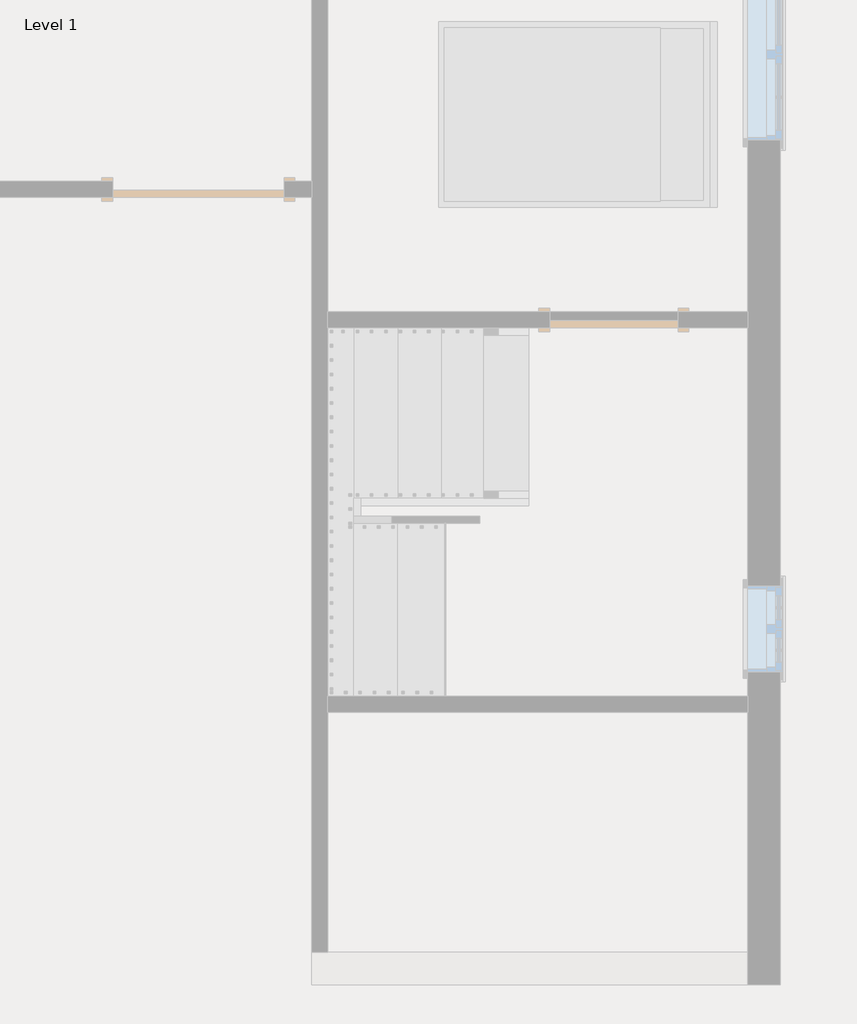
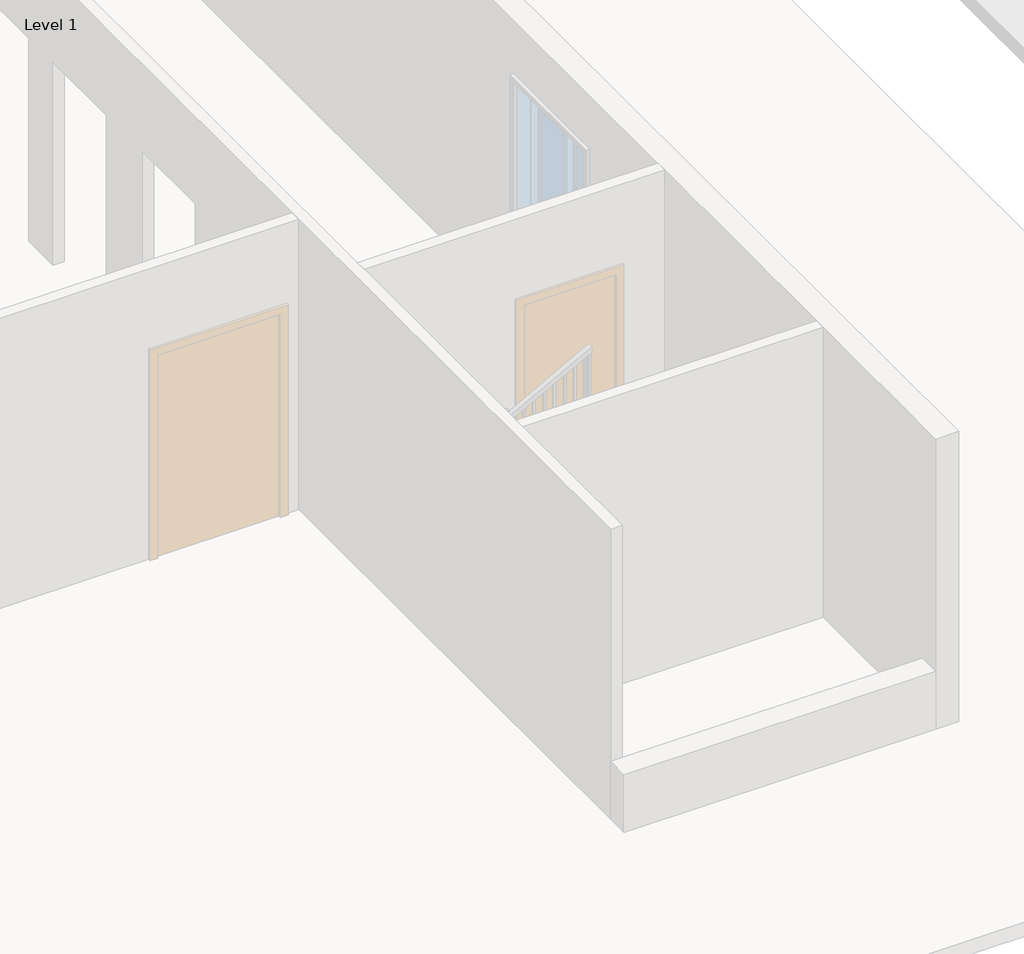
# One storey, part 6 of 7: 2 railings.
"""IFC4 building model written with IfcOpenShell, lengths in millimetres."""

from ifc_helpers import new_model, si_unit, frame, origin, place, context, project, spatial, polyline, outline, extrude, faceted_brep, element, save

model = new_model("IFC4")

# Units and contexts
model_context = context("Model", 3, world=origin())
ifc_project = project(units=[si_unit("LENGTHUNIT", "METRE", prefix="MILLI")], contexts=[model_context])

# Site, building, storey
site = spatial("IfcSite", under=ifc_project)
building = spatial("IfcBuilding", under=site)
storey = spatial("IfcBuildingStorey", under=building, Name="Level 1", Elevation=0.0)

# Railings
placement = place(None, origin())
element("IfcRailing", 1, ObjectType="Handrail - Rectangular", at=placement, inside=storey, context=model_context, shape_type="SolidModel", body=[
    faceted_brep([(7105.1820958, 5435.6, 1083.7333333), (7105.1820958, 5435.6, 1025.8977421), (7105.1820958, 5486.4, 1025.8977421), (7105.1820958, 5486.4, 1083.7333333), (5860.5820958, 5435.6, 1761.0666667), (5847.654197, 5435.6, 1710.2666667), (5847.654197, 5486.4, 1710.2666667), (5860.5820958, 5486.4, 1761.0666667), (5727.7, 5435.6, 1761.0666667), (5727.7, 5435.6, 1710.2666667), (5676.9, 5486.4, 1710.2666667), (5676.9, 5486.4, 1761.0666667), (5727.7, 2997.2, 1761.0666667), (5727.7, 2946.4, 1710.2666667), (5676.9, 2946.4, 1710.2666667), (5676.9, 2997.2, 1761.0666667), (5727.7, 2997.2, 1899.5526009), (5727.7, 2946.4, 1848.7526009), (5676.9, 2946.4, 1848.7526009), (5676.9, 2997.2, 1899.5526009), (5727.7, 2921.0, 1899.5526009), (5727.7, 2921.0, 1848.7526009), (5676.9, 2870.2, 1848.7526009), (5676.9, 2870.2, 1899.5526009), (5803.9, 2921.0, 1899.5526009), (5816.8278988, 2921.0, 1848.7526009), (5816.8278988, 2870.2, 1848.7526009), (5803.9, 2870.2, 1899.5526009), (7105.1820958, 2921.0, 2607.7333333), (7105.1820958, 2870.2, 2607.7333333), (7105.1820958, 2870.2, 2549.8977421), (7105.1820958, 2921.0, 2549.8977421)], [[[0, 1, 2, 3]], [[1, 0, 4, 5]], [[2, 1, 5, 6]], [[3, 2, 6, 7]], [[0, 3, 7, 4]], [[5, 4, 8, 9]], [[6, 5, 9, 10]], [[7, 6, 10, 11]], [[4, 7, 11, 8]], [[9, 8, 12, 13]], [[10, 9, 13, 14]], [[11, 10, 14, 15]], [[8, 11, 15, 12]], [[13, 12, 16, 17]], [[14, 13, 17, 18]], [[15, 14, 18, 19]], [[12, 15, 19, 16]], [[17, 16, 20, 21]], [[18, 17, 21, 22]], [[19, 18, 22, 23]], [[16, 19, 23, 20]], [[21, 20, 24, 25]], [[22, 21, 25, 26]], [[23, 22, 26, 27]], [[20, 23, 27, 24]], [[28, 29, 30, 31]], [[25, 24, 28, 31]], [[26, 25, 31, 30]], [[27, 26, 30, 29]], [[24, 27, 29, 28]]]),
    extrude(outline(polyline([(2510.4108873, 7032.625), (2500.0435403, 7013.575), (1524.0, 7013.575), (1524.0, 7032.625), (2510.4108873, 7032.625)])), frame((0.0, 2886.075, 0.0), z_axis=(0.0, 1.0, 0.0), x_axis=(0.0, 0.0, 1.0)), (0.0, 0.0, 1.0), 19.05),
    extrude(outline(polyline([(2455.1183703, 6931.025), (2444.7510233, 6911.975), (1524.0, 6911.975), (1524.0, 6931.025), (2455.1183703, 6931.025)])), frame((0.0, 2886.075, 0.0), z_axis=(0.0, 1.0, 0.0), x_axis=(0.0, 0.0, 1.0)), (0.0, 0.0, 1.0), 19.05),
    extrude(outline(polyline([(2399.8258533, 6829.425), (2389.4585063, 6810.375), (1524.0, 6810.375), (1524.0, 6829.425), (2399.8258533, 6829.425)])), frame((0.0, 2886.075, 0.0), z_axis=(0.0, 1.0, 0.0), x_axis=(0.0, 0.0, 1.0)), (0.0, 0.0, 1.0), 19.05),
    extrude(outline(polyline([(2344.5333363, 6727.825), (2334.1659893, 6708.775), (1354.6666667, 6708.775), (1354.6666667, 6727.825), (2344.5333363, 6727.825)])), frame((0.0, 2886.075, 0.0), z_axis=(0.0, 1.0, 0.0), x_axis=(0.0, 0.0, 1.0)), (0.0, 0.0, 1.0), 19.05),
    extrude(outline(polyline([(2289.2408192, 6626.225), (2278.8734723, 6607.175), (1354.6666667, 6607.175), (1354.6666667, 6626.225), (2289.2408192, 6626.225)])), frame((0.0, 2886.075, 0.0), z_axis=(0.0, 1.0, 0.0), x_axis=(0.0, 0.0, 1.0)), (0.0, 0.0, 1.0), 19.05),
    extrude(outline(polyline([(2233.9483022, 6524.625), (2223.5809553, 6505.575), (1354.6666667, 6505.575), (1354.6666667, 6524.625), (2233.9483022, 6524.625)])), frame((0.0, 2886.075, 0.0), z_axis=(0.0, 1.0, 0.0), x_axis=(0.0, 0.0, 1.0)), (0.0, 0.0, 1.0), 19.05),
    extrude(outline(polyline([(2178.6557852, 6423.025), (2168.2884383, 6403.975), (1185.3333333, 6403.975), (1185.3333333, 6423.025), (2178.6557852, 6423.025)])), frame((0.0, 2886.075, 0.0), z_axis=(0.0, 1.0, 0.0), x_axis=(0.0, 0.0, 1.0)), (0.0, 0.0, 1.0), 19.05),
    extrude(outline(polyline([(2123.3632682, 6321.425), (2112.9959213, 6302.375), (1185.3333333, 6302.375), (1185.3333333, 6321.425), (2123.3632682, 6321.425)])), frame((0.0, 2886.075, 0.0), z_axis=(0.0, 1.0, 0.0), x_axis=(0.0, 0.0, 1.0)), (0.0, 0.0, 1.0), 19.05),
    extrude(outline(polyline([(2068.0707512, 6219.825), (2057.7034043, 6200.775), (1185.3333333, 6200.775), (1185.3333333, 6219.825), (2068.0707512, 6219.825)])), frame((0.0, 2886.075, 0.0), z_axis=(0.0, 1.0, 0.0), x_axis=(0.0, 0.0, 1.0)), (0.0, 0.0, 1.0), 19.05),
    extrude(outline(polyline([(2012.7782342, 6118.225), (2002.4108873, 6099.175), (1016.0, 6099.175), (1016.0, 6118.225), (2012.7782342, 6118.225)])), frame((0.0, 2886.075, 0.0), z_axis=(0.0, 1.0, 0.0), x_axis=(0.0, 0.0, 1.0)), (0.0, 0.0, 1.0), 19.05),
    extrude(outline(polyline([(1957.4857172, 6016.625), (1947.1183703, 5997.575), (1016.0, 5997.575), (1016.0, 6016.625), (1957.4857172, 6016.625)])), frame((0.0, 2886.075, 0.0), z_axis=(0.0, 1.0, 0.0), x_axis=(0.0, 0.0, 1.0)), (0.0, 0.0, 1.0), 19.05),
    extrude(outline(polyline([(1902.1932002, 5915.025), (1891.8258533, 5895.975), (1016.0, 5895.975), (1016.0, 5915.025), (1902.1932002, 5915.025)])), frame((0.0, 2886.075, 0.0), z_axis=(0.0, 1.0, 0.0), x_axis=(0.0, 0.0, 1.0)), (0.0, 0.0, 1.0), 19.05),
    extrude(outline(polyline([(1846.9006832, 5813.425), (1836.5333363, 5794.375), (846.6666667, 5794.375), (846.6666667, 5813.425), (1846.9006832, 5813.425)])), frame((0.0, 2886.075, 0.0), z_axis=(0.0, 1.0, 0.0), x_axis=(0.0, 0.0, 1.0)), (0.0, 0.0, 1.0), 19.05),
    extrude(outline(polyline([(5692.775, 2930.525), (5711.825, 2930.525), (5711.825, 2911.475), (5692.775, 2911.475), (5692.775, 2930.525)])), frame((0.0, 0.0, 846.6666667), z_axis=(0.0, 0.0, 1.0), x_axis=(1.0, 0.0, 0.0)), (0.0, 0.0, 1.0), 1002.0859343),
    extrude(outline(polyline([(5692.775, 3032.125), (5711.825, 3032.125), (5711.825, 3013.075), (5692.775, 3013.075), (5692.775, 3032.125)])), frame((0.0, 0.0, 846.6666667), z_axis=(0.0, 0.0, 1.0), x_axis=(1.0, 0.0, 0.0)), (0.0, 0.0, 1.0), 863.6),
    extrude(outline(polyline([(5692.775, 3133.725), (5711.825, 3133.725), (5711.825, 3114.675), (5692.775, 3114.675), (5692.775, 3133.725)])), frame((0.0, 0.0, 846.6666667), z_axis=(0.0, 0.0, 1.0), x_axis=(1.0, 0.0, 0.0)), (0.0, 0.0, 1.0), 863.6),
    extrude(outline(polyline([(5692.775, 3235.325), (5711.825, 3235.325), (5711.825, 3216.275), (5692.775, 3216.275), (5692.775, 3235.325)])), frame((0.0, 0.0, 846.6666667), z_axis=(0.0, 0.0, 1.0), x_axis=(1.0, 0.0, 0.0)), (0.0, 0.0, 1.0), 863.6),
    extrude(outline(polyline([(5692.775, 3336.925), (5711.825, 3336.925), (5711.825, 3317.875), (5692.775, 3317.875), (5692.775, 3336.925)])), frame((0.0, 0.0, 846.6666667), z_axis=(0.0, 0.0, 1.0), x_axis=(1.0, 0.0, 0.0)), (0.0, 0.0, 1.0), 863.6),
    extrude(outline(polyline([(5692.775, 3438.525), (5711.825, 3438.525), (5711.825, 3419.475), (5692.775, 3419.475), (5692.775, 3438.525)])), frame((0.0, 0.0, 846.6666667), z_axis=(0.0, 0.0, 1.0), x_axis=(1.0, 0.0, 0.0)), (0.0, 0.0, 1.0), 863.6),
    extrude(outline(polyline([(5692.775, 3540.125), (5711.825, 3540.125), (5711.825, 3521.075), (5692.775, 3521.075), (5692.775, 3540.125)])), frame((0.0, 0.0, 846.6666667), z_axis=(0.0, 0.0, 1.0), x_axis=(1.0, 0.0, 0.0)), (0.0, 0.0, 1.0), 863.6),
    extrude(outline(polyline([(5692.775, 3641.725), (5711.825, 3641.725), (5711.825, 3622.675), (5692.775, 3622.675), (5692.775, 3641.725)])), frame((0.0, 0.0, 846.6666667), z_axis=(0.0, 0.0, 1.0), x_axis=(1.0, 0.0, 0.0)), (0.0, 0.0, 1.0), 863.6),
    extrude(outline(polyline([(5692.775, 3743.325), (5711.825, 3743.325), (5711.825, 3724.275), (5692.775, 3724.275), (5692.775, 3743.325)])), frame((0.0, 0.0, 846.6666667), z_axis=(0.0, 0.0, 1.0), x_axis=(1.0, 0.0, 0.0)), (0.0, 0.0, 1.0), 863.6),
    extrude(outline(polyline([(5692.775, 3844.925), (5711.825, 3844.925), (5711.825, 3825.875), (5692.775, 3825.875), (5692.775, 3844.925)])), frame((0.0, 0.0, 846.6666667), z_axis=(0.0, 0.0, 1.0), x_axis=(1.0, 0.0, 0.0)), (0.0, 0.0, 1.0), 863.6),
    extrude(outline(polyline([(5692.775, 3946.525), (5711.825, 3946.525), (5711.825, 3927.475), (5692.775, 3927.475), (5692.775, 3946.525)])), frame((0.0, 0.0, 846.6666667), z_axis=(0.0, 0.0, 1.0), x_axis=(1.0, 0.0, 0.0)), (0.0, 0.0, 1.0), 863.6),
    extrude(outline(polyline([(5692.775, 4048.125), (5711.825, 4048.125), (5711.825, 4029.075), (5692.775, 4029.075), (5692.775, 4048.125)])), frame((0.0, 0.0, 846.6666667), z_axis=(0.0, 0.0, 1.0), x_axis=(1.0, 0.0, 0.0)), (0.0, 0.0, 1.0), 863.6),
    extrude(outline(polyline([(5692.775, 4149.725), (5711.825, 4149.725), (5711.825, 4130.675), (5692.775, 4130.675), (5692.775, 4149.725)])), frame((0.0, 0.0, 846.6666667), z_axis=(0.0, 0.0, 1.0), x_axis=(1.0, 0.0, 0.0)), (0.0, 0.0, 1.0), 863.6),
    extrude(outline(polyline([(5692.775, 4251.325), (5711.825, 4251.325), (5711.825, 4232.275), (5692.775, 4232.275), (5692.775, 4251.325)])), frame((0.0, 0.0, 846.6666667), z_axis=(0.0, 0.0, 1.0), x_axis=(1.0, 0.0, 0.0)), (0.0, 0.0, 1.0), 863.6),
    extrude(outline(polyline([(5692.775, 4352.925), (5711.825, 4352.925), (5711.825, 4333.875), (5692.775, 4333.875), (5692.775, 4352.925)])), frame((0.0, 0.0, 846.6666667), z_axis=(0.0, 0.0, 1.0), x_axis=(1.0, 0.0, 0.0)), (0.0, 0.0, 1.0), 863.6),
    extrude(outline(polyline([(5692.775, 4454.525), (5711.825, 4454.525), (5711.825, 4435.475), (5692.775, 4435.475), (5692.775, 4454.525)])), frame((0.0, 0.0, 846.6666667), z_axis=(0.0, 0.0, 1.0), x_axis=(1.0, 0.0, 0.0)), (0.0, 0.0, 1.0), 863.6),
    extrude(outline(polyline([(5692.775, 4556.125), (5711.825, 4556.125), (5711.825, 4537.075), (5692.775, 4537.075), (5692.775, 4556.125)])), frame((0.0, 0.0, 846.6666667), z_axis=(0.0, 0.0, 1.0), x_axis=(1.0, 0.0, 0.0)), (0.0, 0.0, 1.0), 863.6),
    extrude(outline(polyline([(5692.775, 4657.725), (5711.825, 4657.725), (5711.825, 4638.675), (5692.775, 4638.675), (5692.775, 4657.725)])), frame((0.0, 0.0, 846.6666667), z_axis=(0.0, 0.0, 1.0), x_axis=(1.0, 0.0, 0.0)), (0.0, 0.0, 1.0), 863.6),
    extrude(outline(polyline([(5692.775, 4759.325), (5711.825, 4759.325), (5711.825, 4740.275), (5692.775, 4740.275), (5692.775, 4759.325)])), frame((0.0, 0.0, 846.6666667), z_axis=(0.0, 0.0, 1.0), x_axis=(1.0, 0.0, 0.0)), (0.0, 0.0, 1.0), 863.6),
    extrude(outline(polyline([(5692.775, 4860.925), (5711.825, 4860.925), (5711.825, 4841.875), (5692.775, 4841.875), (5692.775, 4860.925)])), frame((0.0, 0.0, 846.6666667), z_axis=(0.0, 0.0, 1.0), x_axis=(1.0, 0.0, 0.0)), (0.0, 0.0, 1.0), 863.6),
    extrude(outline(polyline([(5692.775, 4962.525), (5711.825, 4962.525), (5711.825, 4943.475), (5692.775, 4943.475), (5692.775, 4962.525)])), frame((0.0, 0.0, 846.6666667), z_axis=(0.0, 0.0, 1.0), x_axis=(1.0, 0.0, 0.0)), (0.0, 0.0, 1.0), 863.6),
    extrude(outline(polyline([(5692.775, 5064.125), (5711.825, 5064.125), (5711.825, 5045.075), (5692.775, 5045.075), (5692.775, 5064.125)])), frame((0.0, 0.0, 846.6666667), z_axis=(0.0, 0.0, 1.0), x_axis=(1.0, 0.0, 0.0)), (0.0, 0.0, 1.0), 863.6),
    extrude(outline(polyline([(5692.775, 5165.725), (5711.825, 5165.725), (5711.825, 5146.675), (5692.775, 5146.675), (5692.775, 5165.725)])), frame((0.0, 0.0, 846.6666667), z_axis=(0.0, 0.0, 1.0), x_axis=(1.0, 0.0, 0.0)), (0.0, 0.0, 1.0), 863.6),
    extrude(outline(polyline([(5692.775, 5267.325), (5711.825, 5267.325), (5711.825, 5248.275), (5692.775, 5248.275), (5692.775, 5267.325)])), frame((0.0, 0.0, 846.6666667), z_axis=(0.0, 0.0, 1.0), x_axis=(1.0, 0.0, 0.0)), (0.0, 0.0, 1.0), 863.6),
    extrude(outline(polyline([(5692.775, 5368.925), (5711.825, 5368.925), (5711.825, 5349.875), (5692.775, 5349.875), (5692.775, 5368.925)])), frame((0.0, 0.0, 846.6666667), z_axis=(0.0, 0.0, 1.0), x_axis=(1.0, 0.0, 0.0)), (0.0, 0.0, 1.0), 863.6),
    extrude(outline(polyline([(5793.9070958, 5470.525), (5793.9070958, 5451.475), (5774.8570958, 5451.475), (5774.8570958, 5470.525), (5793.9070958, 5470.525)])), frame((0.0, 0.0, 846.6666667), z_axis=(0.0, 0.0, 1.0), x_axis=(1.0, 0.0, 0.0)), (0.0, 0.0, 1.0), 863.6),
    extrude(outline(polyline([(1684.2242727, 5895.5070958), (1694.5916197, 5876.4570958), (677.3333333, 5876.4570958), (677.3333333, 5895.5070958), (1684.2242727, 5895.5070958)])), frame((0.0, 5451.475, 0.0), z_axis=(0.0, 1.0, 0.0), x_axis=(0.0, 0.0, 1.0)), (0.0, 0.0, 1.0), 19.05),
    extrude(outline(polyline([(1628.9317557, 5997.1070958), (1639.2991027, 5978.0570958), (677.3333333, 5978.0570958), (677.3333333, 5997.1070958), (1628.9317557, 5997.1070958)])), frame((0.0, 5451.475, 0.0), z_axis=(0.0, 1.0, 0.0), x_axis=(0.0, 0.0, 1.0)), (0.0, 0.0, 1.0), 19.05),
    extrude(outline(polyline([(1573.6392387, 6098.7070958), (1584.0065857, 6079.6570958), (677.3333333, 6079.6570958), (677.3333333, 6098.7070958), (1573.6392387, 6098.7070958)])), frame((0.0, 5451.475, 0.0), z_axis=(0.0, 1.0, 0.0), x_axis=(0.0, 0.0, 1.0)), (0.0, 0.0, 1.0), 19.05),
    extrude(outline(polyline([(1518.3467217, 6200.3070958), (1528.7140687, 6181.2570958), (508.0, 6181.2570958), (508.0, 6200.3070958), (1518.3467217, 6200.3070958)])), frame((0.0, 5451.475, 0.0), z_axis=(0.0, 1.0, 0.0), x_axis=(0.0, 0.0, 1.0)), (0.0, 0.0, 1.0), 19.05),
    extrude(outline(polyline([(1463.0542047, 6301.9070958), (1473.4215517, 6282.8570958), (508.0, 6282.8570958), (508.0, 6301.9070958), (1463.0542047, 6301.9070958)])), frame((0.0, 5451.475, 0.0), z_axis=(0.0, 1.0, 0.0), x_axis=(0.0, 0.0, 1.0)), (0.0, 0.0, 1.0), 19.05),
    extrude(outline(polyline([(1407.7616877, 6403.5070958), (1418.1290347, 6384.4570958), (508.0, 6384.4570958), (508.0, 6403.5070958), (1407.7616877, 6403.5070958)])), frame((0.0, 5451.475, 0.0), z_axis=(0.0, 1.0, 0.0), x_axis=(0.0, 0.0, 1.0)), (0.0, 0.0, 1.0), 19.05),
    extrude(outline(polyline([(1352.4691707, 6505.1070958), (1362.8365176, 6486.0570958), (338.6666667, 6486.0570958), (338.6666667, 6505.1070958), (1352.4691707, 6505.1070958)])), frame((0.0, 5451.475, 0.0), z_axis=(0.0, 1.0, 0.0), x_axis=(0.0, 0.0, 1.0)), (0.0, 0.0, 1.0), 19.05),
    extrude(outline(polyline([(1297.1766537, 6606.7070958), (1307.5440006, 6587.6570958), (338.6666667, 6587.6570958), (338.6666667, 6606.7070958), (1297.1766537, 6606.7070958)])), frame((0.0, 5451.475, 0.0), z_axis=(0.0, 1.0, 0.0), x_axis=(0.0, 0.0, 1.0)), (0.0, 0.0, 1.0), 19.05),
    extrude(outline(polyline([(1241.8841367, 6708.3070958), (1252.2514836, 6689.2570958), (338.6666667, 6689.2570958), (338.6666667, 6708.3070958), (1241.8841367, 6708.3070958)])), frame((0.0, 5451.475, 0.0), z_axis=(0.0, 1.0, 0.0), x_axis=(0.0, 0.0, 1.0)), (0.0, 0.0, 1.0), 19.05),
    extrude(outline(polyline([(1186.5916197, 6809.9070958), (1196.9589666, 6790.8570958), (169.3333333, 6790.8570958), (169.3333333, 6809.9070958), (1186.5916197, 6809.9070958)])), frame((0.0, 5451.475, 0.0), z_axis=(0.0, 1.0, 0.0), x_axis=(0.0, 0.0, 1.0)), (0.0, 0.0, 1.0), 19.05),
    extrude(outline(polyline([(1131.2991027, 6911.5070958), (1141.6664496, 6892.4570958), (169.3333333, 6892.4570958), (169.3333333, 6911.5070958), (1131.2991027, 6911.5070958)])), frame((0.0, 5451.475, 0.0), z_axis=(0.0, 1.0, 0.0), x_axis=(0.0, 0.0, 1.0)), (0.0, 0.0, 1.0), 19.05),
    extrude(outline(polyline([(1076.0065857, 7013.1070958), (1086.3739326, 6994.0570958), (169.3333333, 6994.0570958), (169.3333333, 7013.1070958), (1076.0065857, 7013.1070958)])), frame((0.0, 5451.475, 0.0), z_axis=(0.0, 1.0, 0.0), x_axis=(0.0, 0.0, 1.0)), (0.0, 0.0, 1.0), 19.05),
    extrude(outline(polyline([(5692.775, 2905.125), (5711.825, 2905.125), (5711.825, 2886.075), (5692.775, 2886.075), (5692.775, 2905.125)])), frame((0.0, 0.0, 846.6666667), z_axis=(0.0, 0.0, 1.0), x_axis=(1.0, 0.0, 0.0)), (0.0, 0.0, 1.0), 1002.0859343),
    extrude(outline(polyline([(5711.825, 5470.525), (5711.825, 5451.475), (5692.775, 5451.475), (5692.775, 5470.525), (5711.825, 5470.525)])), frame((0.0, 0.0, 846.6666667), z_axis=(0.0, 0.0, 1.0), x_axis=(1.0, 0.0, 0.0)), (0.0, 0.0, 1.0), 863.6),
    extrude(outline(polyline([(2549.8977421, 7105.1820958), (2539.5303952, 7086.1320958), (1524.0, 7086.1320958), (1524.0, 7105.1820958), (2549.8977421, 7105.1820958)])), frame((0.0, 2886.075, 0.0), z_axis=(0.0, 1.0, 0.0), x_axis=(0.0, 0.0, 1.0)), (0.0, 0.0, 1.0), 19.05),
    extrude(outline(polyline([(1025.8977421, 7105.1820958), (1036.2650891, 7086.1320958), (169.3333333, 7086.1320958), (169.3333333, 7105.1820958), (1025.8977421, 7105.1820958)])), frame((0.0, 5451.475, 0.0), z_axis=(0.0, 1.0, 0.0), x_axis=(0.0, 0.0, 1.0)), (0.0, 0.0, 1.0), 19.05),
])
element("IfcRailing", 2, ObjectType="Handrail - Rectangular", at=placement, inside=storey, context=model_context, shape_type="SolidModel", body=[
    faceted_brep([(7105.1820958, 4274.6882626, 1083.7333333), (7105.1820958, 4274.6882626, 1025.8977421), (7105.1820958, 4325.4882626, 1025.8977421), (7105.1820958, 4325.4882626, 1083.7333333), (5936.7820958, 4274.6882626, 1719.5972789), (5885.9820958, 4274.6882626, 1689.4079462), (5885.9820958, 4325.4882626, 1689.4079462), (5936.7820958, 4325.4882626, 1719.5972789), (5936.7820958, 4274.6882626, 1761.0666667), (5885.9820958, 4274.6882626, 1710.2666667), (5885.9820958, 4325.4882626, 1710.2666667), (5936.7820958, 4325.4882626, 1761.0666667), (5860.5820958, 4274.6882626, 1761.0666667), (5860.5820958, 4274.6882626, 1710.2666667), (5809.7820958, 4325.4882626, 1710.2666667), (5809.7820958, 4325.4882626, 1761.0666667), (5860.5820958, 4198.4882626, 1761.0666667), (5860.5820958, 4198.4882626, 1710.2666667), (5809.7820958, 4198.4882626, 1710.2666667), (5809.7820958, 4198.4882626, 1761.0666667), (5860.5820958, 4173.0882626, 1761.0666667), (5860.5820958, 4122.2882626, 1710.2666667), (5809.7820958, 4122.2882626, 1710.2666667), (5809.7820958, 4173.0882626, 1761.0666667), (5860.5820958, 4173.0882626, 1971.8693878), (5860.5820958, 4122.2882626, 1921.0693878), (5809.7820958, 4122.2882626, 1921.0693878), (5809.7820958, 4173.0882626, 1971.8693878), (5860.5820958, 4096.8882626, 1971.8693878), (5860.5820958, 4096.8882626, 1921.0693878), (5809.7820958, 4046.0882626, 1921.0693878), (5809.7820958, 4046.0882626, 1971.8693878), (5936.7820958, 4096.8882626, 1971.8693878), (5949.7099946, 4096.8882626, 1921.0693878), (5949.7099946, 4046.0882626, 1921.0693878), (5936.7820958, 4046.0882626, 1971.8693878), (7105.1820958, 4096.8882626, 2607.7333333), (7105.1820958, 4046.0882626, 2607.7333333), (7105.1820958, 4046.0882626, 2549.8977421), (7105.1820958, 4096.8882626, 2549.8977421)], [[[0, 1, 2, 3]], [[1, 0, 4, 5]], [[2, 1, 5, 6]], [[3, 2, 6, 7]], [[0, 3, 7, 4]], [[5, 4, 8, 9]], [[6, 5, 9, 10]], [[7, 6, 10, 11]], [[4, 7, 11, 8]], [[9, 8, 12, 13]], [[10, 9, 13, 14]], [[11, 10, 14, 15]], [[8, 11, 15, 12]], [[13, 12, 16, 17]], [[14, 13, 17, 18]], [[15, 14, 18, 19]], [[12, 15, 19, 16]], [[17, 16, 20, 21]], [[18, 17, 21, 22]], [[19, 18, 22, 23]], [[16, 19, 23, 20]], [[21, 20, 24, 25]], [[22, 21, 25, 26]], [[23, 22, 26, 27]], [[20, 23, 27, 24]], [[25, 24, 28, 29]], [[26, 25, 29, 30]], [[27, 26, 30, 31]], [[24, 27, 31, 28]], [[29, 28, 32, 33]], [[30, 29, 33, 34]], [[31, 30, 34, 35]], [[28, 31, 35, 32]], [[36, 37, 38, 39]], [[33, 32, 36, 39]], [[34, 33, 39, 38]], [[35, 34, 38, 37]], [[32, 35, 37, 36]]]),
    extrude(outline(polyline([(2517.0678102, 7044.8570958), (1524.0, 7044.8570958), (1524.0, 7063.9070958), (2527.4351571, 7063.9070958), (2517.0678102, 7044.8570958)])), frame((0.0, 4061.9632626, 0.0), z_axis=(0.0, 1.0, 0.0), x_axis=(0.0, 0.0, 1.0)), (0.0, 0.0, 1.0), 19.05),
    extrude(outline(polyline([(2461.7752932, 6943.2570958), (1524.0, 6943.2570958), (1524.0, 6962.3070958), (2472.1426401, 6962.3070958), (2461.7752932, 6943.2570958)])), frame((0.0, 4061.9632626, 0.0), z_axis=(0.0, 1.0, 0.0), x_axis=(0.0, 0.0, 1.0)), (0.0, 0.0, 1.0), 19.05),
    extrude(outline(polyline([(2406.4827761, 6841.6570958), (1524.0, 6841.6570958), (1524.0, 6860.7070958), (2416.8501231, 6860.7070958), (2406.4827761, 6841.6570958)])), frame((0.0, 4061.9632626, 0.0), z_axis=(0.0, 1.0, 0.0), x_axis=(0.0, 0.0, 1.0)), (0.0, 0.0, 1.0), 19.05),
    extrude(outline(polyline([(2351.1902591, 6740.0570958), (1354.6666667, 6740.0570958), (1354.6666667, 6759.1070958), (2361.5576061, 6759.1070958), (2351.1902591, 6740.0570958)])), frame((0.0, 4061.9632626, 0.0), z_axis=(0.0, 1.0, 0.0), x_axis=(0.0, 0.0, 1.0)), (0.0, 0.0, 1.0), 19.05),
    extrude(outline(polyline([(2295.8977421, 6638.4570958), (1354.6666667, 6638.4570958), (1354.6666667, 6657.5070958), (2306.2650891, 6657.5070958), (2295.8977421, 6638.4570958)])), frame((0.0, 4061.9632626, 0.0), z_axis=(0.0, 1.0, 0.0), x_axis=(0.0, 0.0, 1.0)), (0.0, 0.0, 1.0), 19.05),
    extrude(outline(polyline([(2240.6052251, 6536.8570958), (1354.6666667, 6536.8570958), (1354.6666667, 6555.9070958), (2250.9725721, 6555.9070958), (2240.6052251, 6536.8570958)])), frame((0.0, 4061.9632626, 0.0), z_axis=(0.0, 1.0, 0.0), x_axis=(0.0, 0.0, 1.0)), (0.0, 0.0, 1.0), 19.05),
    extrude(outline(polyline([(2185.3127081, 6435.2570958), (1185.3333333, 6435.2570958), (1185.3333333, 6454.3070958), (2195.6800551, 6454.3070958), (2185.3127081, 6435.2570958)])), frame((0.0, 4061.9632626, 0.0), z_axis=(0.0, 1.0, 0.0), x_axis=(0.0, 0.0, 1.0)), (0.0, 0.0, 1.0), 19.05),
    extrude(outline(polyline([(2130.0201911, 6333.6570958), (1185.3333333, 6333.6570958), (1185.3333333, 6352.7070958), (2140.3875381, 6352.7070958), (2130.0201911, 6333.6570958)])), frame((0.0, 4061.9632626, 0.0), z_axis=(0.0, 1.0, 0.0), x_axis=(0.0, 0.0, 1.0)), (0.0, 0.0, 1.0), 19.05),
    extrude(outline(polyline([(2074.7276741, 6232.0570958), (1185.3333333, 6232.0570958), (1185.3333333, 6251.1070958), (2085.095021, 6251.1070958), (2074.7276741, 6232.0570958)])), frame((0.0, 4061.9632626, 0.0), z_axis=(0.0, 1.0, 0.0), x_axis=(0.0, 0.0, 1.0)), (0.0, 0.0, 1.0), 19.05),
    extrude(outline(polyline([(2019.4351571, 6130.4570958), (1016.0, 6130.4570958), (1016.0, 6149.5070958), (2029.802504, 6149.5070958), (2019.4351571, 6130.4570958)])), frame((0.0, 4061.9632626, 0.0), z_axis=(0.0, 1.0, 0.0), x_axis=(0.0, 0.0, 1.0)), (0.0, 0.0, 1.0), 19.05),
    extrude(outline(polyline([(1964.1426401, 6028.8570958), (1016.0, 6028.8570958), (1016.0, 6047.9070958), (1974.509987, 6047.9070958), (1964.1426401, 6028.8570958)])), frame((0.0, 4061.9632626, 0.0), z_axis=(0.0, 1.0, 0.0), x_axis=(0.0, 0.0, 1.0)), (0.0, 0.0, 1.0), 19.05),
    extrude(outline(polyline([(1908.8501231, 5927.2570958), (1016.0, 5927.2570958), (1016.0, 5946.3070958), (1919.21747, 5946.3070958), (1908.8501231, 5927.2570958)])), frame((0.0, 4061.9632626, 0.0), z_axis=(0.0, 1.0, 0.0), x_axis=(0.0, 0.0, 1.0)), (0.0, 0.0, 1.0), 19.05),
    extrude(outline(polyline([(5844.7070958, 4106.4132626), (5844.7070958, 4087.3632626), (5825.6570958, 4087.3632626), (5825.6570958, 4106.4132626), (5844.7070958, 4106.4132626)])), frame((0.0, 0.0, 846.6666667), z_axis=(0.0, 0.0, 1.0), x_axis=(1.0, 0.0, 0.0)), (0.0, 0.0, 1.0), 1074.4027211),
    extrude(outline(polyline([(5844.7070958, 4208.0132626), (5844.7070958, 4188.9632626), (5825.6570958, 4188.9632626), (5825.6570958, 4208.0132626), (5844.7070958, 4208.0132626)])), frame((0.0, 0.0, 846.6666667), z_axis=(0.0, 0.0, 1.0), x_axis=(1.0, 0.0, 0.0)), (0.0, 0.0, 1.0), 863.6),
    extrude(outline(polyline([(5895.5070958, 4290.5632626), (5876.4570958, 4290.5632626), (5876.4570958, 4309.6132626), (5895.5070958, 4309.6132626), (5895.5070958, 4290.5632626)])), frame((0.0, 0.0, 677.3333333), z_axis=(0.0, 0.0, 1.0), x_axis=(1.0, 0.0, 0.0)), (0.0, 0.0, 1.0), 1032.9333333),
    extrude(outline(polyline([(1639.2991027, 5978.0570958), (677.3333333, 5978.0570958), (677.3333333, 5997.1070958), (1628.9317557, 5997.1070958), (1639.2991027, 5978.0570958)])), frame((0.0, 4290.5632626, 0.0), z_axis=(0.0, 1.0, 0.0), x_axis=(0.0, 0.0, 1.0)), (0.0, 0.0, 1.0), 19.05),
    extrude(outline(polyline([(1584.0065857, 6079.6570958), (677.3333333, 6079.6570958), (677.3333333, 6098.7070958), (1573.6392387, 6098.7070958), (1584.0065857, 6079.6570958)])), frame((0.0, 4290.5632626, 0.0), z_axis=(0.0, 1.0, 0.0), x_axis=(0.0, 0.0, 1.0)), (0.0, 0.0, 1.0), 19.05),
    extrude(outline(polyline([(1528.7140687, 6181.2570958), (508.0, 6181.2570958), (508.0, 6200.3070958), (1518.3467217, 6200.3070958), (1528.7140687, 6181.2570958)])), frame((0.0, 4290.5632626, 0.0), z_axis=(0.0, 1.0, 0.0), x_axis=(0.0, 0.0, 1.0)), (0.0, 0.0, 1.0), 19.05),
    extrude(outline(polyline([(1473.4215517, 6282.8570958), (508.0, 6282.8570958), (508.0, 6301.9070958), (1463.0542047, 6301.9070958), (1473.4215517, 6282.8570958)])), frame((0.0, 4290.5632626, 0.0), z_axis=(0.0, 1.0, 0.0), x_axis=(0.0, 0.0, 1.0)), (0.0, 0.0, 1.0), 19.05),
    extrude(outline(polyline([(1418.1290347, 6384.4570958), (508.0, 6384.4570958), (508.0, 6403.5070958), (1407.7616877, 6403.5070958), (1418.1290347, 6384.4570958)])), frame((0.0, 4290.5632626, 0.0), z_axis=(0.0, 1.0, 0.0), x_axis=(0.0, 0.0, 1.0)), (0.0, 0.0, 1.0), 19.05),
    extrude(outline(polyline([(1362.8365176, 6486.0570958), (338.6666667, 6486.0570958), (338.6666667, 6505.1070958), (1352.4691707, 6505.1070958), (1362.8365176, 6486.0570958)])), frame((0.0, 4290.5632626, 0.0), z_axis=(0.0, 1.0, 0.0), x_axis=(0.0, 0.0, 1.0)), (0.0, 0.0, 1.0), 19.05),
    extrude(outline(polyline([(1307.5440006, 6587.6570958), (338.6666667, 6587.6570958), (338.6666667, 6606.7070958), (1297.1766537, 6606.7070958), (1307.5440006, 6587.6570958)])), frame((0.0, 4290.5632626, 0.0), z_axis=(0.0, 1.0, 0.0), x_axis=(0.0, 0.0, 1.0)), (0.0, 0.0, 1.0), 19.05),
    extrude(outline(polyline([(1252.2514836, 6689.2570958), (338.6666667, 6689.2570958), (338.6666667, 6708.3070958), (1241.8841367, 6708.3070958), (1252.2514836, 6689.2570958)])), frame((0.0, 4290.5632626, 0.0), z_axis=(0.0, 1.0, 0.0), x_axis=(0.0, 0.0, 1.0)), (0.0, 0.0, 1.0), 19.05),
    extrude(outline(polyline([(1196.9589666, 6790.8570958), (169.3333333, 6790.8570958), (169.3333333, 6809.9070958), (1186.5916197, 6809.9070958), (1196.9589666, 6790.8570958)])), frame((0.0, 4290.5632626, 0.0), z_axis=(0.0, 1.0, 0.0), x_axis=(0.0, 0.0, 1.0)), (0.0, 0.0, 1.0), 19.05),
    extrude(outline(polyline([(1141.6664496, 6892.4570958), (169.3333333, 6892.4570958), (169.3333333, 6911.5070958), (1131.2991027, 6911.5070958), (1141.6664496, 6892.4570958)])), frame((0.0, 4290.5632626, 0.0), z_axis=(0.0, 1.0, 0.0), x_axis=(0.0, 0.0, 1.0)), (0.0, 0.0, 1.0), 19.05),
    extrude(outline(polyline([(1086.3739326, 6994.0570958), (169.3333333, 6994.0570958), (169.3333333, 7013.1070958), (1076.0065857, 7013.1070958), (1086.3739326, 6994.0570958)])), frame((0.0, 4290.5632626, 0.0), z_axis=(0.0, 1.0, 0.0), x_axis=(0.0, 0.0, 1.0)), (0.0, 0.0, 1.0), 19.05),
    extrude(outline(polyline([(5844.7070958, 4081.0132626), (5844.7070958, 4061.9632626), (5825.6570958, 4061.9632626), (5825.6570958, 4081.0132626), (5844.7070958, 4081.0132626)])), frame((0.0, 0.0, 846.6666667), z_axis=(0.0, 0.0, 1.0), x_axis=(1.0, 0.0, 0.0)), (0.0, 0.0, 1.0), 1074.4027211),
    extrude(outline(polyline([(5844.7070958, 4290.5632626), (5825.6570958, 4290.5632626), (5825.6570958, 4309.6132626), (5844.7070958, 4309.6132626), (5844.7070958, 4290.5632626)])), frame((0.0, 0.0, 846.6666667), z_axis=(0.0, 0.0, 1.0), x_axis=(1.0, 0.0, 0.0)), (0.0, 0.0, 1.0), 863.6),
    extrude(outline(polyline([(2539.5303952, 7086.1320958), (1524.0, 7086.1320958), (1524.0, 7105.1820958), (2549.8977421, 7105.1820958), (2539.5303952, 7086.1320958)])), frame((0.0, 4061.9632626, 0.0), z_axis=(0.0, 1.0, 0.0), x_axis=(0.0, 0.0, 1.0)), (0.0, 0.0, 1.0), 19.05),
    extrude(outline(polyline([(1036.2650891, 7086.1320958), (169.3333333, 7086.1320958), (169.3333333, 7105.1820958), (1025.8977421, 7105.1820958), (1036.2650891, 7086.1320958)])), frame((0.0, 4290.5632626, 0.0), z_axis=(0.0, 1.0, 0.0), x_axis=(0.0, 0.0, 1.0)), (0.0, 0.0, 1.0), 19.05),
])

save(model, "model.ifc")

# Revit data of these elements
# Type "Handrail - Rectangular"
#   Assembly Code = "C2010400"
#   built-in parameter 1008612 = 0.0416667 (stored number, unit not read)
#   built-in parameter 1008611 = 0.0416667 (stored number, unit not read)
#   built-in parameter 1008609 = 0.333333 (stored number, unit not read)
#   built-in parameter 1008604 = 0.166667 (stored number, unit not read)
#   built-in parameter 1008603 = 0.166667 (stored number, unit not read)
#   Railing Height = 3' - 0"
#   built-in parameter 1008630 = 2
#   built-in parameter 1008610 = 2
#   built-in parameter 1008618 = Baluster - Square : 3/4"
# Elements 1, 2 (IfcRailing, "Handrail - Rectangular")
#   Phase Created = New Construction
